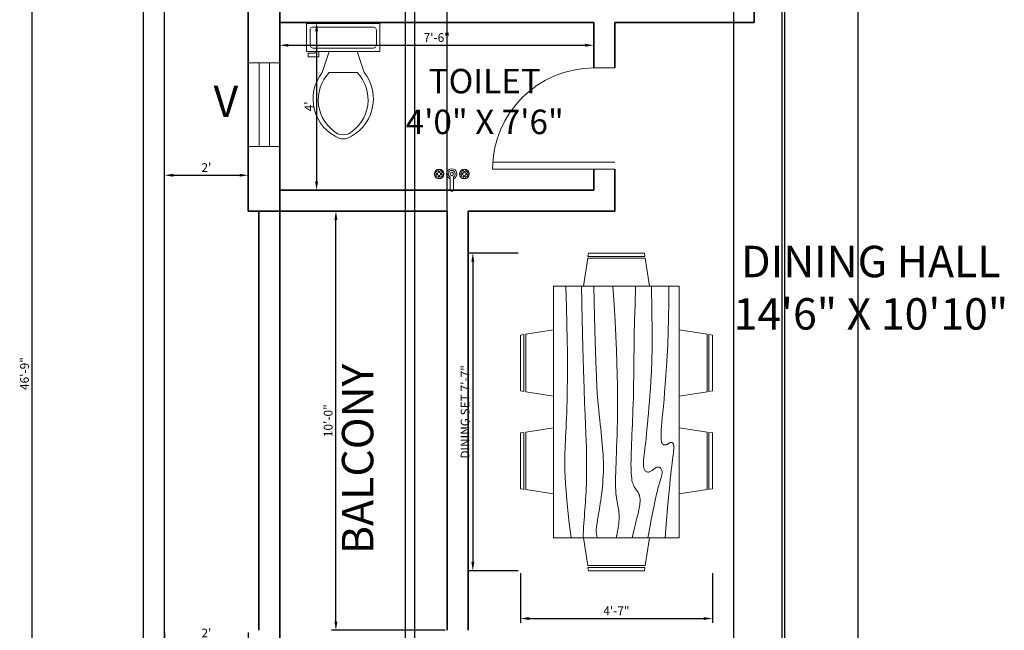
# Model space of a CAD drawing. Units: inches. Extents: x 1879 to 2382, y 1769 to 2461.
# Tile 2 of 5: x 1881 to 2163, y 2015 to 2190. Entities that reach past the tile are written whole.
import ezdxf

# ---------------------------------------------------------------- set-up
doc = ezdxf.new("R2010")
doc.units = ezdxf.units.IN
for name, color, linetype, lineweight in [('A-ANNO-DIMS', 2, 'Continuous', 18), ('A-ANNO-TEXT', 3, 'Continuous', 18), ('A-AREA-IDEN', 7, 'Continuous', 18), ('A-DOOR', 3, 'Continuous', 18), ('A-FLOR-FIXT', 9, 'Continuous', 18), ('A-FURN', 9, 'Continuous', 18), ('A-GLAZ', 4, 'Continuous', 18), ('A-WALL', 7, 'Continuous', 35), ('C-PROP', 1, 'Continuous', 25)]:
    doc.layers.add(name, color=color, linetype=linetype, lineweight=lineweight)
doc.styles.get("Standard").update_dxf_attribs({"font": 'arial.ttf'})
doc.dimstyles.new('ISO-25', dxfattribs={"dimtxt": 2.5, "dimasz": 2.5, "dimexe": 1.25, "dimexo": 0.625, "dimtad": 1, "dimlunit": 4, "dimtxsty": 'Standard', "dimcen": 2.5, "dimadec": 0, "dimazin": 0, "dimtfac": 1, "dimtmove": 0, "dimatfit": 3, "dimfxl": 1, "dimarcsym": 0})

# ---------------------------------------------------------------- blocks, each defined once
blk = doc.blocks.new('*U4')
for p, q in [((9.5, -6), (9.5, -2)), ((-8, -8.5), (-8, -8)), ((-7, -8), (-7, -9.5)), ((-4, -8), (-6, -14)), ((4, -8), (6, -14)), ((-10, -8.5), (-8, -8.5)), ((-10, -9.5), (-10, -8.5)), ((-7, -9.5), (-10, -9.5)), ((4, -14), (-4, -14))]:
    blk.add_line(p, q)
blk.add_lwpolyline([(10.5, -8), (10.5, 0), (-10.5, 0), (-10.5, -8)], close=True)
for points in [[(-9.5, -2), (-9.5, -6)], [(8.5, -1), (-8.5, -1)], [(-8.5, -7), (8.5, -7)]]:
    blk.add_lwpolyline(points)
for centre, radius, start, end in [((-8.62, -1.88), 0.884, 81.8699, 188.1301), ((8.62, -1.88), 0.884, 351.8699, 98.1301), ((-8.62, -6.12), 0.884, 171.8699, 278.1301), ((8.62, -6.12), 0.884, 261.8699, 8.1301), ((3.52, -21.58), 12.17, 141.4691, 247.9714), ((4.2, -21.82), 11.33, 136.3677, 238.9468), ((-3.52, -21.58), 12.17, 292.0284, 38.5307), ((-4.2, -21.82), 11.33, 301.053, 43.6321), ((0, -27.88), 4, 245.7318, 294.2682), ((0, -29), 4, 254.8605, 285.1395)]:
    blk.add_arc(centre, radius, start, end)
blk = doc.blocks.new('Dining Set - 36 x 72 in.')
for p, q in [((-22.2343, 26.00059), (-23.4847, 17.99762)), ((-22.2304, 26), (-5.7608, 26)), ((-22, 27.5), (-22.1562, 26.50042)), ((-5.8416, 26.5), (-22.1534, 26.5)), ((-22, 27.5), (-6, 27.5)), ((-5.8437, 26.49966), (-6, 27.5)), ((-4.5152, 17.99762), (-5.7655, 25.99926)), ((5.7657, 26.00059), (4.5153, 17.99762)), ((5.7696, 26), (22.2392, 26)), ((6, 27.5), (5.8438, 26.50042)), ((22.1584, 26.5), (5.8466, 26.5)), ((6, 27.5), (22, 27.5)), ((22.1563, 26.49966), (22, 27.5)), ((23.4848, 17.99762), (22.2345, 25.99926)), ((36, 18), (-36, 18)), ((-36, 18), (-36, -18)), ((36, -18), (36, 18)), ((-44.0006, 8.23428), (-35.9976, 9.48474)), ((44.0006, 8.23428), (35.9976, 9.48474)), ((-45.5, 8), (-44.5004, 8.15617)), ((-45.5, 8), (-45.5, -8)), ((-44.5, -8.15843), (-44.5, 8.15338)), ((-44, 8.23041), (-44, -8.23915)), ((44, 8.23041), (44, -8.23915)), ((44.5, -8.15843), (44.5, 8.15338)), ((45.5, 8), (44.5005, 8.15617)), ((45.5, 8), (45.5, -8)), ((-44.4997, -8.15631), (-45.5, -8)), ((-35.9976, -9.48476), (-43.9993, -8.2345)), ((35.9976, -9.48476), (43.9993, -8.2345)), ((44.4997, -8.15631), (45.5, -8)), ((-36, -18), (36, -18)), ((-22.2343, -26.0006), (-23.4847, -17.99762)), ((-4.5152, -17.99762), (-5.7655, -25.99928)), ((5.7657, -26.0006), (4.5153, -17.99762)), ((23.4848, -17.99762), (22.2345, -25.99928)), ((-22.2304, -26), (-5.7608, -26)), ((-22, -27.5), (-22.1562, -26.50044)), ((-5.8416, -26.5), (-22.1534, -26.5)), ((-22, -27.5), (-6, -27.5)), ((-5.8437, -26.49967), (-6, -27.5)), ((5.7696, -26), (22.2392, -26)), ((6, -27.5), (5.8438, -26.50044)), ((22.1584, -26.5), (5.8466, -26.5)), ((6, -27.5), (22, -27.5)), ((22.1563, -26.49967), (22, -27.5))]:
    blk.add_line(p, q)
for points in [[(-36, 15), (-31.1772, 14.97754), (-26.8079, 14.91406), (-22.8538, 14.81543), (-19.276, 14.6875), (-16.0362, 14.53613), (-13.0957, 14.36718), (-10.4159, 14.18652), (-7.9583, 14), (-5.6904, 13.81315), (-3.6035, 13.63021), (-1.6954, 13.45508), (0.0365, 13.29166), (1.5945, 13.14388), (2.9811, 13.01562), (4.1988, 12.9108), (5.25, 12.83333), (6.1393, 12.78613), (6.8802, 12.76823), (7.4883, 12.77767), (7.9792, 12.8125), (8.3685, 12.87077), (8.6719, 12.95052), (8.9049, 13.0498), (9.0833, 13.16666), (9.2205, 13.29899), (9.3216, 13.44401), (9.3895, 13.59879), (9.4271, 13.76041), (9.4373, 13.92594), (9.4232, 14.09245), (9.3875, 14.257), (9.3333, 14.41666), (9.2638, 14.56917), (9.1836, 14.71484), (9.0975, 14.85465), (9.0104, 14.98958), (8.9272, 15.1206), (8.8529, 15.2487), (8.7922, 15.37483), (8.75, 15.5), (8.7305, 15.62467), (8.7344, 15.74739), (8.7617, 15.86621), (8.8125, 15.97916), (8.8867, 16.08431), (8.9844, 16.17968), (9.1055, 16.26334), (9.25, 16.33333), (9.4189, 16.38802), (9.6172, 16.42708), (9.8506, 16.45052), (10.125, 16.45833), (10.4463, 16.45052), (10.8203, 16.42708), (11.2529, 16.38802), (11.75, 16.33333), (12.3184, 16.26318), (12.9694, 16.17838), (13.7151, 16.07991), (14.5677, 15.96875), (15.5395, 15.84586), (16.6426, 15.71224), (17.8893, 15.56884), (19.2917, 15.41666), (20.859, 15.25667), (22.5879, 15.08984), (24.4721, 14.91715), (26.5052, 14.73958), (28.6809, 14.5581), (30.9929, 14.3737), (33.4347, 14.18733), (36, 14)], [(-36, 10), (-28.9766, 10.14274), (-23.1725, 10.20442), (-18.4241, 10.19775), (-14.5677, 10.13541), (-11.4399, 10.03011), (-8.877, 9.89453), (-6.7154, 9.74137), (-4.7917, 9.58333), (-2.9698, 9.43082), (-1.2246, 9.28515), (0.4415, 9.14534), (2.026, 9.01041), (3.5266, 8.87939), (4.9408, 8.7513), (6.266, 8.62516), (7.5, 8.5), (8.6411, 8.37549), (9.6914, 8.2539), (10.6538, 8.13818), (11.5312, 8.03125), (12.3267, 7.93603), (13.043, 7.85547), (13.6831, 7.79248), (14.25, 7.75), (14.7471, 7.7303), (15.1797, 7.73307), (15.5537, 7.75732), (15.875, 7.80208), (16.1494, 7.86637), (16.3828, 7.94922), (16.5811, 8.04964), (16.75, 8.16666), (16.8944, 8.29915), (17.0143, 8.44531), (17.1089, 8.60319), (17.1771, 8.77083), (17.218, 8.94629), (17.2305, 9.1276), (17.2137, 9.31282), (17.1667, 9.5), (17.0895, 9.6875), (16.987, 9.875), (16.8649, 10.0625), (16.7292, 10.25), (16.5856, 10.4375), (16.4401, 10.625), (16.2985, 10.8125), (16.1667, 11), (16.05, 11.18733), (15.9518, 11.3737), (15.8752, 11.5581), (15.8229, 11.73958), (15.798, 11.91715), (15.8034, 12.08984), (15.842, 12.25667), (15.9167, 12.41666), (16.0295, 12.56836), (16.1784, 12.70833), (16.3605, 12.83268), (16.5729, 12.9375), (16.8127, 13.01888), (17.0768, 13.07291), (17.3625, 13.0957), (17.6667, 13.08333), (17.9894, 13.03312), (18.3418, 12.94726), (18.7382, 12.82918), (19.1927, 12.68229), (19.7195, 12.51001), (20.3327, 12.31575), (21.0465, 12.10294), (21.875, 11.875), (22.8357, 11.63354), (23.959, 11.37304), (25.2786, 11.08618), (26.8282, 10.76562), (28.6414, 10.40405), (30.752, 9.99414), (33.1936, 9.52856), (36, 9)], [(-36, 5.5), (-30.7157, 5.3348), (-26.069, 5.20963), (-21.9946, 5.11767), (-18.4271, 5.05208), (-15.3009, 5.00602), (-12.5508, 4.97265), (-10.1112, 4.94515), (-7.9167, 4.91666), (-5.909, 4.88167), (-4.0586, 4.83984), (-2.3429, 4.79215), (-0.7396, 4.73958), (0.7739, 4.6831), (2.22, 4.6237), (3.6213, 4.56233), (5, 4.5), (6.373, 4.43782), (7.7344, 4.3776), (9.0723, 4.32129), (10.375, 4.27083), (11.6309, 4.22819), (12.8281, 4.19531), (13.9551, 4.17415), (15, 4.16666), (15.954, 4.17448), (16.819, 4.19791), (17.6001, 4.23698), (18.3021, 4.29166), (18.9299, 4.36198), (19.4883, 4.44791), (19.9823, 4.54948), (20.4167, 4.66666), (20.7969, 4.79899), (21.1302, 4.94401), (21.4245, 5.09879), (21.6875, 5.26041), (21.9271, 5.42594), (22.1511, 5.59245), (22.3672, 5.757), (22.5834, 5.91666), (22.8065, 6.06868), (23.0404, 6.21093), (23.2879, 6.34147), (23.5521, 6.45833), (23.8358, 6.55957), (24.142, 6.64323), (24.4735, 6.70735), (24.8334, 6.75), (25.2235, 6.76969), (25.642, 6.76692), (26.0858, 6.74267), (26.5521, 6.69791), (27.0379, 6.63362), (27.5404, 6.55078), (28.0565, 6.45036), (28.5834, 6.33333), (29.1242, 6.19987), (29.7071, 6.04687), (30.3661, 5.87044), (31.1354, 5.66666), (32.0493, 5.43164), (33.142, 5.16146), (34.4475, 4.85221), (36, 4.5)], [(-36, -1), (-30.7915, -0.6591), (-26.0195, -0.38216), (-21.6519, -0.16284), (-17.6563, 0.00521), (-14.0005, 0.12833), (-10.6523, 0.21289), (-7.5796, 0.26522), (-4.75, 0.29166), (-2.134, 0.29793), (0.2878, 0.28711), (2.5317, 0.26163), (4.6146, 0.22396), (6.5529, 0.17651), (8.3633, 0.12174), (10.0623, 0.06209), (11.6667, 0), (13.1899, -0.06201), (14.6341, -0.1211), (15.9982, -0.17432), (17.2813, -0.21875), (18.4823, -0.25147), (19.6003, -0.26953), (20.6343, -0.27002), (21.5834, -0.25), (22.4481, -0.20768), (23.2357, -0.14584), (23.9549, -0.06836), (24.6146, 0.02083), (25.2235, 0.11784), (25.7904, 0.21875), (26.3241, 0.31966), (26.8334, 0.41666), (27.3265, 0.50618), (27.8099, 0.58593), (28.2894, 0.65397), (28.7709, 0.70833), (29.2601, 0.74707), (29.763, 0.76823), (30.2855, 0.76985), (30.8334, 0.75), (31.4088, 0.70784), (31.9994, 0.64713), (32.589, 0.57275), (33.1615, 0.48958), (33.7008, 0.4025), (34.1908, 0.3164), (34.6153, 0.23616), (34.9584, 0.16666), (35.2099, 0.11165), (35.3848, 0.07031), (35.504, 0.04069), (35.5886, 0.02083), (35.6594, 0.00879), (35.7377, 0.0026), (35.8442, 0.00032), (36, 0)], [(-36, -6.5), (-27.1843, -6.31267), (-20.084, -6.1263), (-14.469, -5.9419), (-10.1094, -5.76042), (-6.7752, -5.58285), (-4.2363, -5.41016), (-2.2629, -5.24333), (-0.625, -5.08334), (0.8708, -4.93099), (2.2715, -4.78646), (3.5872, -4.64974), (4.8281, -4.52084), (6.0046, -4.39974), (7.127, -4.28646), (8.2053, -4.18099), (9.25, -4.08334), (10.2705, -3.99382), (11.2734, -3.91407), (12.2647, -3.84603), (13.25, -3.79167), (14.2354, -3.75293), (15.2266, -3.73177), (16.2295, -3.73015), (17.25, -3.75), (18.2912, -3.79248), (19.3451, -3.85547), (20.4009, -3.93604), (21.4479, -4.03125), (22.4754, -4.13819), (23.4727, -4.25391), (24.4289, -4.37549), (25.3334, -4.5), (26.1785, -4.62492), (26.9694, -4.74935), (27.7145, -4.87281), (28.4219, -4.99479), (29.1, -5.11483), (29.7572, -5.23242), (30.4016, -5.34709), (31.0417, -5.45834), (31.6837, -5.56437), (32.3262, -5.65821), (32.9658, -5.73153), (33.599, -5.77604), (34.2224, -5.78345), (34.8327, -5.74545), (35.4264, -5.65373), (36, -5.5)], [(-36, -10), (-26.4022, -9.81299), (-18.4675, -9.62891), (-11.9839, -9.45069), (-6.7396, -9.28125), (-2.5226, -9.12354), (0.8789, -8.98047), (3.6769, -8.85498), (6.0833, -8.75), (8.2767, -8.66765), (10.3021, -8.60677), (12.1712, -8.56543), (13.8958, -8.54167), (15.4876, -8.53353), (16.9583, -8.53907), (18.3197, -8.55632), (19.5834, -8.58334), (20.7616, -8.61841), (21.8685, -8.66081), (22.9188, -8.71004), (23.9271, -8.76563), (24.9081, -8.82707), (25.8763, -8.89388), (26.8465, -8.96558), (27.8334, -9.04167), (28.8474, -9.12118), (29.8828, -9.20117), (30.93, -9.27824), (31.9792, -9.34896), (33.0205, -9.40991), (34.0443, -9.45768), (35.0407, -9.48885), (36, -9.5)], [(-36, -14.5), (-30.0881, -14.33513), (-25.0332, -14.21224), (-20.7312, -14.12647), (-17.0781, -14.07292), (-13.97, -14.04671), (-11.3027, -14.04297), (-8.9724, -14.05681), (-6.875, -14.08334), (-4.9224, -14.11833), (-3.0905, -14.16016), (-1.3709, -14.20785), (0.2448, -14.26042), (1.7647, -14.3169), (3.1973, -14.3763), (4.5507, -14.43767), (5.8333, -14.5), (7.0554, -14.5621), (8.235, -14.62175), (9.3922, -14.67652), (10.5469, -14.72396), (11.7192, -14.76164), (12.929, -14.78711), (14.1965, -14.79794), (15.5417, -14.79167), (16.9933, -14.76424), (18.6152, -14.70508), (20.4804, -14.60197), (22.6615, -14.44271), (25.2312, -14.21509), (28.2624, -13.9069), (31.8277, -13.50594), (36, -13)]]:
    blk.add_lwpolyline(points)
blk = doc.blocks.new('Faucet - Bathroom top')
for p, q in [((-4.107, 0.125), (-4.375, 0.125)), ((-3.75, 0.4788), (-3.75, 0.75)), ((-3.5, 0.482), (-3.5, 0.75)), ((-3.1461, 0.125), (-2.875, 0.125)), ((3.143, 0.125), (2.875, 0.125)), ((3.5, 0.4788), (3.5, 0.75)), ((3.75, 0.482), (3.75, 0.75)), ((4.1039, 0.125), (4.375, 0.125)), ((-4.1039, -0.125), (-4.375, -0.125)), ((-3.75, -0.4821), (-3.75, -0.75)), ((-3.5, -0.4789), (-3.5, -0.75)), ((-3.143, -0.125), (-2.875, -0.125)), ((-0.5, -0.8639), (-0.5, -4.5)), ((0.5, -4.5), (0.5, -0.8631)), ((3.1461, -0.125), (2.875, -0.125)), ((3.5, -0.4821), (3.5, -0.75)), ((3.75, -0.4789), (3.75, -0.75)), ((4.107, -0.125), (4.375, -0.125))]:
    blk.add_line(p, q)
for centre, radius in [((-3.625, 0), 1.375), ((-4.625, 0), 0.2795), ((-3.625, 0), 0.5), ((-3.625, 1), 0.2795), ((-2.625, 0), 0.2795), ((0, 0), 0.5), ((3.625, 0), 1.375), ((2.625, 0), 0.2795), ((3.625, 0), 0.5), ((3.625, 1), 0.2795), ((4.625, 0), 0.2795), ((-3.625, -1), 0.2795), ((3.625, -1), 0.2795)]:
    blk.add_circle(centre, radius)
for centre, radius, start, end in [((-3.625, 0), 1, 105.2407, 164.2093), ((-3.625, 0), 1, 16.44125, 74.07887), ((0, 0), 1.5, 289.6514, 250.3603), ((0, 0), 1, 300.3431, 239.7554), ((3.625, 0), 1, 106.12, 164.0884), ((3.625, 0), 1, 16.23422, 73.90469), ((-3.625, 0), 1, 196.2342, 253.9047), ((-3.625, 0), 1, 286.12, 344.0884), ((3.625, 0), 1, 196.4413, 254.0789), ((3.625, 0), 1, 285.2407, 344.2093), ((0, -4.5), 0.5, 180, 0)]:
    blk.add_arc(centre, radius, start, end)
blk = doc.blocks.new('*D20')
at = {"layer": 'A-ANNO-DIMS', "color": 0, "lineweight": -2, "transparency": 16777216}
for p, q in [((1922.34, 2145.26), (1922.34, 2146.71)), ((1924.84, 2145.46), (1943.84, 2145.46)), ((1946.34, 2145.26), (1946.34, 2146.71))]:
    blk.add_line(p, q, dxfattribs=at)
at = {"layer": 'A-ANNO-DIMS', "color": 0, "transparency": 16777216}
for points in [[(1924.84, 2145.88), (1924.84, 2145.05), (1922.34, 2145.46)], [(1943.84, 2145.88), (1943.84, 2145.05), (1946.34, 2145.46)]]:
    blk.add_solid(points, dxfattribs=at)
at = {"layer": 'Defpoints', "color": 0, "transparency": 16777216}
for p in [(1922.34, 2144.63), (1946.34, 2145.46), (1946.34, 2144.63)]:
    blk.add_point(p, dxfattribs=at)
at = {"layer": 'A-ANNO-DIMS', "color": 0, "transparency": 16777216, "insert": (1934.34, 2147.34), "char_height": 2.5, "attachment_point": 5}
blk.add_mtext("2'", dxfattribs=at)
blk = doc.blocks.new('*D21')
at = {"layer": 'A-ANNO-DIMS', "color": 0, "lineweight": -2, "transparency": 16777216}
for p, q in [((1922.34, 2014.56), (1922.34, 2010.95)), ((1946.34, 2014.56), (1946.34, 2010.95)), ((1943.84, 2012.2), (1924.84, 2012.2))]:
    blk.add_line(p, q, dxfattribs=at)
at = {"layer": 'A-ANNO-DIMS', "color": 0, "transparency": 16777216}
for points in [[(1924.84, 2012.62), (1924.84, 2011.79), (1922.34, 2012.2)], [(1943.84, 2012.62), (1943.84, 2011.79), (1946.34, 2012.2)]]:
    blk.add_solid(points, dxfattribs=at)
at = {"layer": 'Defpoints', "color": 0, "transparency": 16777216}
for p in [(1922.34, 2015.18), (1946.34, 2015.18), (1922.34, 2012.2)]:
    blk.add_point(p, dxfattribs=at)
at = {"layer": 'A-ANNO-DIMS', "color": 0, "transparency": 16777216, "insert": (1934.34, 2014.08), "char_height": 2.5, "attachment_point": 5}
blk.add_mtext("2'", dxfattribs=at)
blk = doc.blocks.new('*D22')
at = {"layer": 'A-ANNO-DIMS', "color": 0, "lineweight": -2, "transparency": 16777216}
for p, q in [((1955.34, 2188.56), (1955.34, 2181.43)), ((2045.34, 2188.56), (2045.34, 2181.43)), ((1957.84, 2182.68), (2042.84, 2182.68))]:
    blk.add_line(p, q, dxfattribs=at)
at = {"layer": 'A-ANNO-DIMS', "color": 0, "transparency": 16777216}
for points in [[(1957.84, 2183.1), (1957.84, 2182.26), (1955.34, 2182.68)], [(2042.84, 2183.1), (2042.84, 2182.26), (2045.34, 2182.68)]]:
    blk.add_solid(points, dxfattribs=at)
at = {"layer": 'Defpoints', "color": 0, "transparency": 16777216}
for p in [(1955.34, 2189.18), (2045.34, 2189.18), (2045.34, 2182.68)]:
    blk.add_point(p, dxfattribs=at)
at = {"layer": 'A-ANNO-DIMS', "color": 0, "transparency": 16777216, "insert": (2000.34, 2184.58), "char_height": 2.5, "attachment_point": 5}
blk.add_mtext('7\'-6"', dxfattribs=at)
blk = doc.blocks.new('*D23')
at = {"layer": 'A-ANNO-DIMS', "color": 0, "lineweight": -2, "transparency": 16777216}
for p, q in [((1955.97, 2189.18), (1967.16, 2189.18)), ((1965.91, 2186.68), (1965.91, 2143.68)), ((1955.97, 2141.18), (1967.16, 2141.18))]:
    blk.add_line(p, q, dxfattribs=at)
at = {"layer": 'A-ANNO-DIMS', "color": 0, "transparency": 16777216}
for points in [[(1965.49, 2186.68), (1966.33, 2186.68), (1965.91, 2189.18)], [(1965.49, 2143.68), (1966.33, 2143.68), (1965.91, 2141.18)]]:
    blk.add_solid(points, dxfattribs=at)
at = {"layer": 'Defpoints', "color": 0, "transparency": 16777216}
for p in [(1955.34, 2189.18), (1955.34, 2141.18), (1965.91, 2141.18)]:
    blk.add_point(p, dxfattribs=at)
at = {"layer": 'A-ANNO-DIMS', "color": 0, "transparency": 16777216, "insert": (1964.03, 2165.18), "char_height": 2.5, "attachment_point": 5, "rotation": 90}
blk.add_mtext("4'", dxfattribs=at)
blk = doc.blocks.new('VENT-24x9')
for p, q in [((24, 9), (0, 9)), ((0, 9), (0, 0)), ((24, 9), (24, 0)), ((24, 6), (0, 6)), ((0, 3), (24, 3)), ((0, 0), (24, 0))]:
    blk.add_line(p, q)
blk = doc.blocks.new('DR-SWING-29')
for p, q in [((27, 6), (27, 35)), ((29, 6), (29, 35)), ((0, 0), (0, 6)), ((27, 6), (27, 0)), ((29, 6), (29, 0))]:
    blk.add_line(p, q)
blk.add_arc((29, 6), 29, 90, 180)
blk = doc.blocks.new('*D45')
at = {"layer": 'A-ANNO-DIMS', "color": 0, "lineweight": -2, "transparency": 16777216}
for p, q in [((2023.71, 2123.2), (2009.43, 2123.2)), ((2010.68, 2120.7), (2010.68, 2034.7)), ((2023.71, 2032.2), (2009.43, 2032.2))]:
    blk.add_line(p, q, dxfattribs=at)
at = {"layer": 'A-ANNO-DIMS', "color": 0, "transparency": 16777216}
for points in [[(2010.27, 2120.7), (2011.1, 2120.7), (2010.68, 2123.2)], [(2010.27, 2034.7), (2011.1, 2034.7), (2010.68, 2032.2)]]:
    blk.add_solid(points, dxfattribs=at)
at = {"layer": 'Defpoints', "color": 0, "transparency": 16777216}
for p in [(2024.33, 2123.2), (2010.68, 2032.2), (2024.33, 2032.2)]:
    blk.add_point(p, dxfattribs=at)
at = {"layer": 'A-ANNO-DIMS', "color": 0, "transparency": 16777216, "insert": (2008.77, 2077.7), "char_height": 2.5, "attachment_point": 5, "rotation": 90}
blk.add_mtext('DINING SET 7\'-7"', dxfattribs=at)
blk = doc.blocks.new('*D46')
at = {"layer": 'A-ANNO-DIMS', "color": 0, "lineweight": -2, "transparency": 16777216}
for p, q in [((2024.33, 2031.57), (2024.33, 2017.3)), ((2079.33, 2031.57), (2079.33, 2017.3)), ((2026.83, 2018.55), (2076.83, 2018.55))]:
    blk.add_line(p, q, dxfattribs=at)
at = {"layer": 'A-ANNO-DIMS', "color": 0, "transparency": 16777216}
for points in [[(2026.83, 2018.96), (2026.83, 2018.13), (2024.33, 2018.55)], [(2076.83, 2018.96), (2076.83, 2018.13), (2079.33, 2018.55)]]:
    blk.add_solid(points, dxfattribs=at)
at = {"layer": 'Defpoints', "color": 0, "transparency": 16777216}
for p in [(2024.33, 2032.2), (2079.33, 2032.2), (2079.33, 2018.55)]:
    blk.add_point(p, dxfattribs=at)
at = {"layer": 'A-ANNO-DIMS', "color": 0, "transparency": 16777216, "insert": (2051.83, 2020.42), "char_height": 2.5, "attachment_point": 5}
blk.add_mtext('4\'-7"', dxfattribs=at)
blk = doc.blocks.new('*D56')
at = {"layer": 'A-ANNO-DIMS', "color": 0, "lineweight": -2, "transparency": 16777216}
for p, q in [((1945.72, 2369.18), (1883.19, 2369.18)), ((1884.44, 1810.68), (1884.44, 2366.68)), ((1945.72, 1808.18), (1883.19, 1808.18))]:
    blk.add_line(p, q, dxfattribs=at)
at = {"layer": 'A-ANNO-DIMS', "color": 0, "transparency": 16777216}
for points in [[(1884.02, 2366.68), (1884.86, 2366.68), (1884.44, 2369.18)], [(1884.02, 1810.68), (1884.86, 1810.68), (1884.44, 1808.18)]]:
    blk.add_solid(points, dxfattribs=at)
at = {"layer": 'Defpoints', "color": 0, "transparency": 16777216}
for p in [(1884.44, 2369.18), (1946.34, 2369.18), (1946.34, 1808.18)]:
    blk.add_point(p, dxfattribs=at)
at = {"layer": 'A-ANNO-DIMS', "color": 0, "transparency": 16777216, "insert": (1882.54, 2088.68), "char_height": 2.5, "attachment_point": 5, "rotation": 90}
blk.add_mtext('46\'-9"', dxfattribs=at)
blk = doc.blocks.new('*D61')
at = {"layer": 'A-ANNO-DIMS', "color": 0, "lineweight": -2, "transparency": 16777216}
for p, q in [((1955.34, 2015.81), (1955.34, 2456.28)), ((1957.84, 2455.03), (2000.84, 2455.03)), ((2003.34, 2015.81), (2003.34, 2456.28))]:
    blk.add_line(p, q, dxfattribs=at)
at = {"layer": 'A-ANNO-DIMS', "color": 0, "transparency": 16777216}
for points in [[(1957.84, 2455.44), (1957.84, 2454.61), (1955.34, 2455.03)], [(2000.84, 2455.44), (2000.84, 2454.61), (2003.34, 2455.03)]]:
    blk.add_solid(points, dxfattribs=at)
at = {"layer": 'Defpoints', "color": 0, "transparency": 16777216}
for p in [(2003.34, 2455.03), (1955.34, 2015.18), (2003.34, 2015.18)]:
    blk.add_point(p, dxfattribs=at)
at = {"layer": 'A-ANNO-DIMS', "color": 0, "transparency": 16777216, "insert": (1979.34, 2456.93), "char_height": 2.5, "attachment_point": 5}
blk.add_mtext('4\'-0"', dxfattribs=at)
blk = doc.blocks.new('*D62')
at = {"layer": 'A-ANNO-DIMS', "color": 0, "lineweight": -2, "transparency": 16777216}
for p, q in [((2099.99, 2354.46), (2099.99, 1769.03)), ((2120.99, 2354.46), (2120.99, 1769.03)), ((2102.49, 1770.28), (2118.49, 1770.28))]:
    blk.add_line(p, q, dxfattribs=at)
at = {"layer": 'A-ANNO-DIMS', "color": 0, "transparency": 16777216}
for points in [[(2102.49, 1770.7), (2102.49, 1769.86), (2099.99, 1770.28)], [(2118.49, 1770.7), (2118.49, 1769.86), (2120.99, 1770.28)]]:
    blk.add_solid(points, dxfattribs=at)
at = {"layer": 'Defpoints', "color": 0, "transparency": 16777216}
for p in [(2099.99, 2355.08), (2120.99, 2355.08), (2120.99, 1770.28)]:
    blk.add_point(p, dxfattribs=at)
at = {"layer": 'A-ANNO-DIMS', "color": 0, "transparency": 16777216, "insert": (2110.49, 1772.18), "char_height": 2.5, "attachment_point": 5}
blk.add_mtext('1\'-9"', dxfattribs=at)
blk = doc.blocks.new('*D65')
at = {"layer": 'A-ANNO-DIMS', "color": 0, "lineweight": -2, "transparency": 16777216}
for p, q in [((1991.34, 1850.81), (1991.34, 2456.28)), ((1993.84, 2455.03), (2096.84, 2455.03)), ((2099.34, 1850.81), (2099.34, 2456.28))]:
    blk.add_line(p, q, dxfattribs=at)
at = {"layer": 'A-ANNO-DIMS', "color": 0, "transparency": 16777216}
for points in [[(1993.84, 2455.44), (1993.84, 2454.61), (1991.34, 2455.03)], [(2096.84, 2455.44), (2096.84, 2454.61), (2099.34, 2455.03)]]:
    blk.add_solid(points, dxfattribs=at)
at = {"layer": 'Defpoints', "color": 0, "transparency": 16777216}
for p in [(2099.34, 2455.03), (1991.34, 1850.18), (2099.34, 1850.18)]:
    blk.add_point(p, dxfattribs=at)
at = {"layer": 'A-ANNO-DIMS', "color": 0, "transparency": 16777216, "insert": (2045.34, 2456.93), "char_height": 2.5, "attachment_point": 5}
blk.add_mtext('9\'-0"', dxfattribs=at)
blk = doc.blocks.new('*D67')
at = {"layer": 'A-ANNO-DIMS', "color": 0, "lineweight": -2, "transparency": 16777216}
for p, q in [((1955.34, 1901.81), (1955.34, 2456.28)), ((1957.84, 2455.03), (1991.58, 2455.03)), ((1994.08, 1901.81), (1994.08, 2456.28))]:
    blk.add_line(p, q, dxfattribs=at)
at = {"layer": 'A-ANNO-DIMS', "color": 0, "transparency": 16777216}
for points in [[(1957.84, 2455.44), (1957.84, 2454.61), (1955.34, 2455.03)], [(1991.58, 2455.44), (1991.58, 2454.61), (1994.08, 2455.03)]]:
    blk.add_solid(points, dxfattribs=at)
at = {"layer": 'Defpoints', "color": 0, "transparency": 16777216}
for p in [(1994.08, 2455.03), (1955.34, 1901.18), (1994.08, 1901.18)]:
    blk.add_point(p, dxfattribs=at)
at = {"layer": 'A-ANNO-DIMS', "color": 0, "transparency": 16777216, "insert": (1974.71, 2456.95), "char_height": 2.5, "attachment_point": 5}
blk.add_mtext('3\'-2 1/2"', dxfattribs=at)
blk = doc.blocks.new('*D71')
at = {"layer": 'A-ANNO-DIMS', "color": 0, "lineweight": -2, "transparency": 16777216}
for p, q in [((1955.34, 2362.56), (1955.34, 1769.03)), ((2085.34, 2362.56), (2085.34, 1769.03)), ((1957.84, 1770.28), (2082.84, 1770.28))]:
    blk.add_line(p, q, dxfattribs=at)
at = {"layer": 'A-ANNO-DIMS', "color": 0, "transparency": 16777216}
for points in [[(1957.84, 1770.7), (1957.84, 1769.86), (1955.34, 1770.28)], [(2082.84, 1770.7), (2082.84, 1769.86), (2085.34, 1770.28)]]:
    blk.add_solid(points, dxfattribs=at)
at = {"layer": 'Defpoints', "color": 0, "transparency": 16777216}
for p in [(1955.34, 2363.18), (2085.34, 2363.18), (2085.34, 1770.28)]:
    blk.add_point(p, dxfattribs=at)
at = {"layer": 'A-ANNO-DIMS', "color": 0, "transparency": 16777216, "insert": (2020.34, 1772.18), "char_height": 2.5, "attachment_point": 5}
blk.add_mtext('10\'-10"', dxfattribs=at)
blk = doc.blocks.new('*D72')
at = {"layer": 'A-ANNO-DIMS', "color": 0, "lineweight": -2, "transparency": 16777216}
for p, q in [((2002.72, 2135.18), (1970.19, 2135.18)), ((1971.44, 2017.68), (1971.44, 2132.68)), ((2002.72, 2015.18), (1970.19, 2015.18))]:
    blk.add_line(p, q, dxfattribs=at)
at = {"layer": 'A-ANNO-DIMS', "color": 0, "transparency": 16777216}
for points in [[(1971.02, 2132.68), (1971.86, 2132.68), (1971.44, 2135.18)], [(1971.02, 2017.68), (1971.86, 2017.68), (1971.44, 2015.18)]]:
    blk.add_solid(points, dxfattribs=at)
at = {"layer": 'Defpoints', "color": 0, "transparency": 16777216}
for p in [(1971.44, 2135.18), (2003.34, 2135.18), (2003.34, 2015.18)]:
    blk.add_point(p, dxfattribs=at)
at = {"layer": 'A-ANNO-DIMS', "color": 0, "transparency": 16777216, "insert": (1969.54, 2075.18), "char_height": 2.5, "attachment_point": 5, "rotation": 90}
blk.add_mtext('10\'-0"', dxfattribs=at)

msp = doc.modelspace()

# ---------------------------------------------------------------- linework, layer by layer
at = {"layer": 'A-WALL'}
for p, q in [((1946.341, 2135.18), (1946.341, 2369.18)), ((2091.341, 2189.18), (2091.341, 2205.18)), ((1955.341, 2189.18), (2045.341, 2189.18)), ((1955.341, 2141.18), (1955.341, 2189.18)), ((2045.341, 2176.18), (2045.341, 2189.18)), ((2051.341, 2189.18), (2091.341, 2189.18)), ((2051.341, 2176.18), (2051.341, 2189.18)), ((2045.341, 2141.18), (2045.341, 2147.18)), ((2045.341, 2141.18), (2045.341, 2147.18)), ((2051.341, 2135.18), (2051.341, 2147.18)), ((1955.341, 2141.18), (2045.341, 2141.18)), ((1955.341, 2135.18), (1946.341, 2135.18)), ((1949.341, 2015.18), (1949.341, 2135.18)), ((1955.341, 2135.18), (2003.341, 2135.18)), ((1955.341, 2015.18), (1955.341, 2135.18)), ((2003.341, 2015.18), (2003.341, 2135.18)), ((2009.341, 2015.18), (2009.341, 2135.18)), ((2009.341, 2135.18), (2051.341, 2135.18))]:
    msp.add_line(p, q, dxfattribs=at)
at = {"layer": 'C-PROP'}
for p, q in [((1916.341, 1802.18), (1916.341, 2402.18)), ((1922.341, 1808.18), (1922.341, 2396.18))]:
    msp.add_line(p, q, dxfattribs=at)

# ---------------------------------------------------------------- block references
at = {"layer": 'A-DOOR', "extrusion": (0, 0, -1), "zscale": -1, "rotation": 269.9999999999994}
msp.add_blockref('DR-SWING-29', (-2051.341, 2176.18), dxfattribs=at)
at = {"layer": 'A-FLOR-FIXT'}
for name, p in [('*U4', (1973.534, 2188.884)), ('Faucet - Bathroom top', (2004.639, 2145.838))]:
    msp.add_blockref(name, p, dxfattribs=at)
at = {"layer": 'A-FURN', "rotation": 270}
msp.add_blockref('Dining Set - 36 x 72 in.', (2051.833, 2077.696), dxfattribs=at)
at = {"layer": 'A-GLAZ', "rotation": 89.99999999999785}
msp.add_blockref('VENT-24x9', (1955.41, 2153.665), dxfattribs=at)

# ---------------------------------------------------------------- texts
at = {"layer": 'A-ANNO-TEXT', "insert": (1883.802, 2171.111), "char_height": 9, "attachment_point": 1}
msp.add_mtext_dynamic_manual_height_columns('\\pxqc;V', width=112.22887, gutter_width=12.5, heights=[0], dxfattribs=at)
at = {"layer": 'A-AREA-IDEN', "attachment_point": 1}
for s, width, insert, char_height in [('\\pxqc;TOILET\\P4\'0" X 7\'6"', 57.18405, (1985.492, 2175.912), 7), ('\\pxqc;DINING HALL\\P14\'6" X 10\'10" ', 85.79731, (2081.839, 2125.27), 9)]:
    msp.add_mtext_dynamic_manual_height_columns(s, width=width, gutter_width=12.5, heights=[0], dxfattribs=dict(at, insert=insert, char_height=char_height))
at = {"layer": 'A-AREA-IDEN', "insert": (1973.166, 2036.979), "char_height": 9, "attachment_point": 1, "rotation": 90}
msp.add_mtext_dynamic_manual_height_columns('BALCONY', width=86.90732, gutter_width=12.5, heights=[0], dxfattribs=at)

# ---------------------------------------------------------------- dimensions: what is measured, and where the dimension line sits
at = {"layer": 'A-ANNO-DIMS'}
for base, p1, p2, override, picture, middle in [((1994.083, 2455.028), (1955.341, 1901.18), (1994.083, 1901.18), {"dimdec": 1, "dimlfac": 1, "dimrnd": 0, "dimzin": 1, "dimdsep": 46, "dimlunit": 4, "dimfrac": 2}, '*D67', (1974.712, 2456.946)), ((2003.341, 2455.028), (1955.341, 2015.18), (2003.341, 2015.18), {"dimdec": 1, "dimlfac": 1, "dimrnd": 0, "dimzin": 1, "dimdsep": 46, "dimlunit": 4, "dimfrac": 2}, '*D61', (1979.341, 2456.929)), ((2099.341, 2455.028), (1991.341, 1850.18), (2099.341, 1850.18), {"dimdec": 1, "dimlfac": 1, "dimrnd": 0, "dimzin": 1, "dimdsep": 46, "dimlunit": 4, "dimfrac": 2}, '*D65', (2045.341, 2456.929)), ((2085.341, 1770.28), (1955.341, 2363.18), (2085.341, 2363.18), {"dimdec": 1, "dimlfac": 1, "dimrnd": 0, "dimzin": 1, "dimdsep": 46, "dimlunit": 4, "dimfrac": 2}, '*D71', (2020.341, 1772.182)), ((2120.987, 1770.28), (2099.987, 2355.082), (2120.987, 2355.082), {"dimdec": 1, "dimlfac": 1, "dimrnd": 0, "dimzin": 1, "dimdsep": 46, "dimlunit": 4, "dimfrac": 2}, '*D62', (2110.487, 1772.182)), ((2045.341, 2182.68), (1955.341, 2189.18), (2045.341, 2189.18), {"dimclrd": 0, "dimclre": 0, "dimclrt": 0}, '*D22', (2000.341, 2184.582)), ((1946.341, 2145.462), (1922.341, 2144.631), (1946.341, 2144.631), {"dimclrd": 0, "dimclre": 0, "dimclrt": 0}, '*D20', (1934.341, 2147.342)), ((2079.333, 2018.546), (2024.333, 2032.196), (2079.333, 2032.196), {"dimdec": 1, "dimlfac": 1, "dimrnd": 0, "dimzin": 1, "dimdsep": 46, "dimlunit": 4, "dimfrac": 2}, '*D46', (2051.833, 2020.421)), ((1922.341, 2012.202), (1946.341, 2015.18), (1922.341, 2015.18), {"dimclrd": 0, "dimclre": 0, "dimclrt": 0}, '*D21', (1934.341, 2014.082))]:
    dim = msp.add_linear_dim(base=base, p1=p1, p2=p2, dimstyle='ISO-25', override=override, dxfattribs=at)
    dim.commit()
    dim.dimension.update_dxf_attribs({"geometry": picture, "text_midpoint": middle})
for base, p1, p2, override, picture, middle in [((1884.441, 2369.18), (1946.341, 1808.18), (1946.341, 2369.18), {"dimdec": 1, "dimlfac": 1, "dimrnd": 0, "dimzin": 1, "dimdsep": 46, "dimlunit": 4, "dimfrac": 2}, '*D56', (1882.54, 2088.68)), ((1965.909, 2141.18), (1955.341, 2189.18), (1955.341, 2141.18), {"dimclrd": 0, "dimclre": 0, "dimclrt": 0}, '*D23', (1964.034, 2165.18)), ((1971.441, 2135.18), (2003.341, 2015.18), (2003.341, 2135.18), {"dimdec": 1, "dimlfac": 1, "dimrnd": 0, "dimzin": 1, "dimdsep": 46, "dimlunit": 4, "dimfrac": 2}, '*D72', (1969.54, 2075.18))]:
    dim = msp.add_linear_dim(base=base, p1=p1, p2=p2, angle=90, dimstyle='ISO-25', override=override, dxfattribs=at)
    dim.commit()
    dim.dimension.update_dxf_attribs({"geometry": picture, "text_midpoint": middle})
dim = msp.add_linear_dim(base=(2010.683, 2032.196), p1=(2024.333, 2123.196), p2=(2024.333, 2032.196), angle=270, text='DINING SET <>', dimstyle='ISO-25', override={"dimdec": 1, "dimlfac": 1, "dimrnd": 0, "dimzin": 1, "dimdsep": 46, "dimlunit": 4, "dimfrac": 2}, dxfattribs=at)
dim.commit()
dim.dimension.update_dxf_attribs({"geometry": '*D45', "text_midpoint": (2008.766, 2077.696)})

doc.saveas('drawing.dxf')
